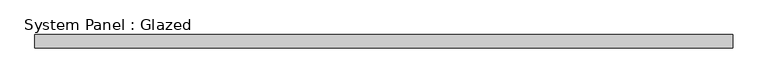
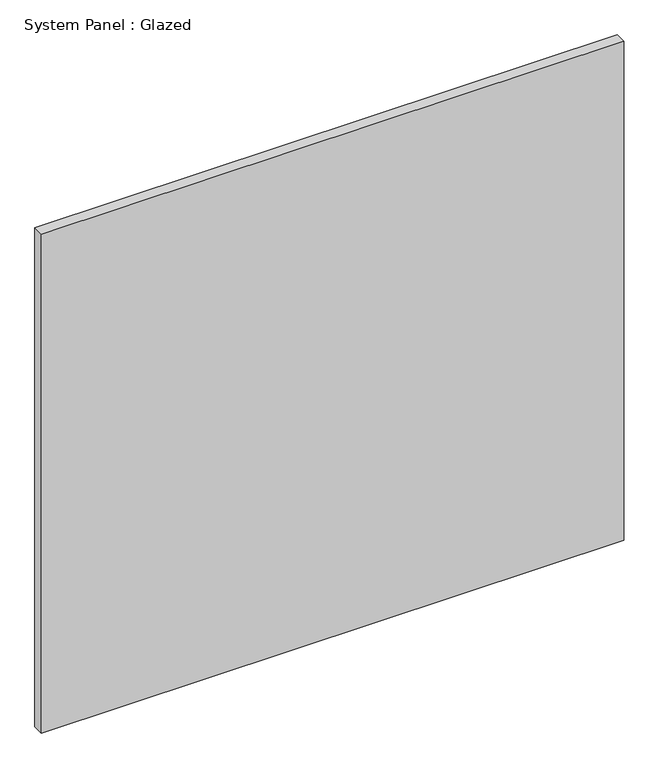
"""IFC4 building model written with IfcOpenShell, lengths in millimetres: plate geometry, System Panel : Glazed."""

from ifc_helpers import new_model, si_unit, origin, origin_with_axes, place, context, project, spatial, polyline, outline, extrude, source, transform, mapped, element, save


def system_panel_glazed_7d767388(model_context):
    return source(origin(), model_context, "Body", "SweptSolid", [
        extrude(outline(polyline([(673.1, 19.05), (-673.1, 19.05), (-673.1, 44.45), (673.1, 44.45), (673.1, 19.05)])), origin_with_axes(), (0.0, 0.0, 1.0), 1219.2),
    ])


if __name__ == "__main__":
    model = new_model("IFC4")
    model_context = context("Model", 3, world=origin())
    ifc_project = project(units=[si_unit("LENGTHUNIT", "METRE", prefix="MILLI")], contexts=[model_context])
    site = spatial("IfcSite", under=ifc_project)
    building = spatial("IfcBuilding", under=site)
    placement = place(None, origin())
    system_panel_glazed_shape = system_panel_glazed_7d767388(model_context)
    element("IfcPlate", 1, ObjectType="System Panel : Glazed", at=placement, inside=building, context=model_context, shape_type="MappedRepresentation", body=[
        mapped(system_panel_glazed_shape, transform((0.0, 0.0, 0.0), x_axis=(1.0, 0.0, 0.0), y_axis=(0.0, 1.0, 0.0), z_axis=(0.0, 0.0, 1.0))),
    ])
    save(model, "model.ifc")

# Revit data of these elements
# Type "System Panel : Glazed"
#   Construction Type Id = "GSP4R"
#   Analytic Construction = "1/8 in Pilkington single glazing"
#   Visual Light Transmittance = 0.9
#   Solar Heat Gain Coefficient = 0.86
#   Heat Transfer Coefficient (U) = 1.18115 BTU/(h·ft²·°F)
# Element 1 (IfcPlate, "System Panel : Glazed")
#   Materials on its faces: "Glass"
# Materials
#   "Glass": class "Glass", colour RGB 0 128 192, transparency 0.75, Description = "Soda Lime Glass", Cost = 0
